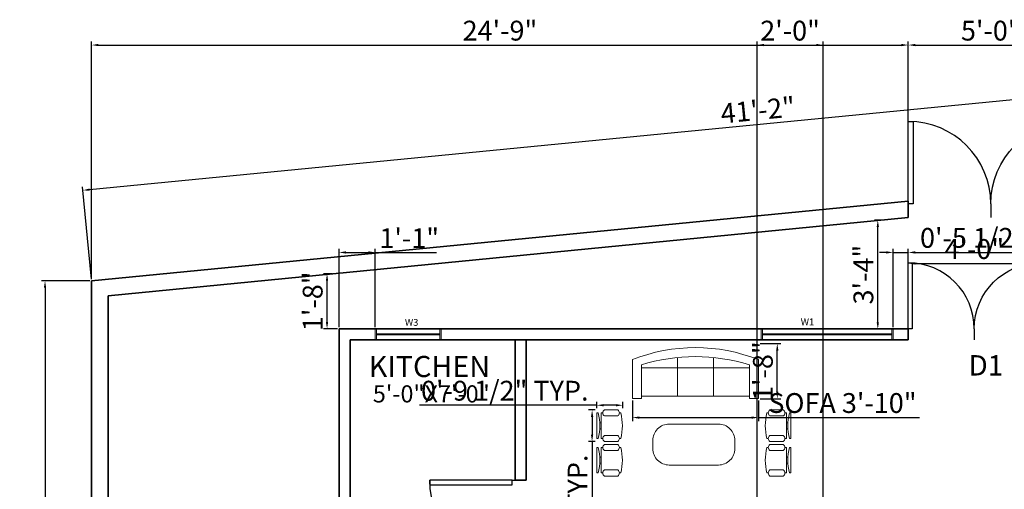
# Model space of a CAD drawing. Units: inches. Extents: x 2165 to 6441, y 2023 to 4425.
# Tile 2 of 4: x 2176 to 2534, y 2281 to 2452. Entities that reach past the tile are written whole.
import ezdxf

# ---------------------------------------------------------------- set-up
doc = ezdxf.new("R2010")
doc.units = ezdxf.units.IN
for name, color, linetype, lineweight in [('A-ANNO-DIMS', 7, 'Continuous', 18), ('A-ANNO-TEXT', 1, 'Continuous', 18), ('A-AREA-IDEN', 1, 'Continuous', 25), ('C-PROP', 7, 'Continuous', 35), ('doors', 5, 'Continuous', 25), ('furniture', 9, 'Continuous', 18), ('walls', 7, 'Continuous', 35), ('windows', 72, 'Continuous', 18)]:
    doc.layers.add(name, color=color, linetype=linetype, lineweight=lineweight)
doc.styles.get("Standard").update_dxf_attribs({"font": 'arial.ttf'})
doc.dimstyles.new('ISO-25', dxfattribs={"dimtxt": 7.203125, "dimasz": 2.5, "dimexe": 1.25, "dimexo": 0.625, "dimtad": 1, "dimdec": 0, "dimlunit": 4, "dimtxsty": 'Standard', "dimcen": 2.5, "dimadec": 0, "dimazin": 0, "dimtfac": 1, "dimtdec": 0, "dimtmove": 0, "dimatfit": 3, "dimfxl": 1, "dimarcsym": 0})

# ---------------------------------------------------------------- blocks, each defined once
blk = doc.blocks.new('*U2')
for p, q in [((0, 0), (0, -5)), ((30, 0), (30, -5))]:
    blk.add_line(p, q)
blk.add_lwpolyline([(0, 0), (0, 30), (1.75, 30), (1.75, 0)], close=True)
blk.add_arc((0, 0), 30, 0, 90)
blk = doc.blocks.new('Sofa - Roundback 7 ft.')
for p, q in [((-36.000027, -34), (-36.000027, -11.4696)), ((-12.00002, -32.4421), (-12.00003, -6.5971)), ((11.99997, -32.4421), (11.99998, -6.5971)), ((35.99998, -34), (35.99998, -11.4696)), ((-35.999844, -13.3819), (35.9998, -13.3819)), ((-36.000027, -32.4421), (35.99998, -32.4421))]:
    blk.add_line(p, q)
for points in [[(-36.000027, -34), (-42.000027, -34), (-42.000027, -8)], [(41.99998, -8), (41.99998, -34), (35.99998, -34)]]:
    blk.add_lwpolyline(points)
for centre, radius, start, end in [((0, -114.25), 114.25, 68.43141, 111.5686), ((-0.00001, -127.1968), 121.1968, 72.72033, 107.2797)]:
    blk.add_arc(centre, radius, start, end)
blk = doc.blocks.new('Chair - Desk')
for p, q in [((-8.5, 0), (-8.5, -1)), ((-8.5, 0), (8.5, 0)), ((8.5, 0), (8.5, -1)), ((-10.5, -5), (-10.5, -14)), ((-8.5, -3), (-8.5, -4)), ((-8.5, -3), (8.5, -3)), ((-6.5, -14), (-6.5, -5)), ((-2, -3), (-2, -1.9355)), ((2, -1.9576), (2, -3)), ((6.5, -5), (6.5, -14)), ((8.5, -3), (8.5, -4)), ((10.5, -14), (10.5, -5)), ((-8.5, -15), (-8.5, -16)), ((8.5, -15), (8.5, -16))]:
    blk.add_line(p, q)
for centre, radius, start, end in [((-8.5, -6.5), 2.5, 36.8699, 143.1301), ((0, 34.625), 36.625, 256.5803, 283.4197), ((8.5, -6.5), 2.5, 36.8699, 143.1301), ((-8.5, -12.5), 2.5, 216.8699, 323.1301), ((0, 19.625), 36.625, 256.5803, 283.4197), ((8.5, -12.5), 2.5, 216.8699, 323.1301)]:
    blk.add_arc(centre, radius, start, end)
blk = doc.blocks.new('*D8')
at = {"layer": 'A-ANNO-DIMS', "color": 0, "lineweight": -2, "transparency": 16777216}
for p, q in [((2693.62, 2405.41), (2690.35, 2438.92)), ((2200.96, 2389.92), (2687.99, 2437.43)), ((2201.62, 2357.41), (2198.35, 2390.92))]:
    blk.add_line(p, q, dxfattribs=at)
at = {"layer": 'A-ANNO-DIMS', "color": 0, "transparency": 16777216}
for points in [[(2687.95, 2437.85), (2688.03, 2437.02), (2690.48, 2437.67)], [(2200.92, 2390.33), (2201, 2389.5), (2198.48, 2389.67)]]:
    blk.add_solid(points, dxfattribs=at)
at = {"layer": 'Defpoints', "color": 0, "transparency": 16777216}
for p in [(2690.48, 2437.67), (2693.68, 2404.78), (2201.68, 2356.78)]:
    blk.add_point(p, dxfattribs=at)
at = {"layer": 'A-ANNO-DIMS', "color": 0, "transparency": 16777216, "insert": (2444.06, 2417.9), "char_height": 7.203, "attachment_point": 5, "rotation": 5.5722}
blk.add_mtext('41\'-2"', dxfattribs=at)
blk = doc.blocks.new('*D10')
at = {"layer": 'A-ANNO-DIMS', "color": 0, "lineweight": -2, "transparency": 16777216}
for p, q in [((2201.06, 2356.78), (2183.49, 2356.78)), ((2184.74, 2354.28), (2184.74, 2059.28)), ((2201.06, 2056.78), (2183.49, 2056.78))]:
    blk.add_line(p, q, dxfattribs=at)
at = {"layer": 'A-ANNO-DIMS', "color": 0, "transparency": 16777216}
for points in [[(2184.32, 2354.28), (2185.15, 2354.28), (2184.74, 2356.78)], [(2184.32, 2059.28), (2185.15, 2059.28), (2184.74, 2056.78)]]:
    blk.add_solid(points, dxfattribs=at)
at = {"layer": 'Defpoints', "color": 0, "transparency": 16777216}
for p in [(2201.68, 2356.78), (2184.74, 2056.78), (2201.68, 2056.78)]:
    blk.add_point(p, dxfattribs=at)
at = {"layer": 'A-ANNO-DIMS', "color": 0, "transparency": 16777216, "insert": (2180.43, 2206.78), "char_height": 7.203, "attachment_point": 5, "rotation": 90}
blk.add_mtext("25'", dxfattribs=at)
blk = doc.blocks.new('*D15')
at = {"layer": 'A-ANNO-DIMS', "color": 0, "lineweight": -2, "transparency": 16777216}
for p, q in [((2289.11, 2359.35), (2286.05, 2359.35)), ((2287.3, 2341.84), (2287.3, 2356.85)), ((2291.06, 2339.34), (2286.05, 2339.34))]:
    blk.add_line(p, q, dxfattribs=at)
at = {"layer": 'A-ANNO-DIMS', "color": 0, "transparency": 16777216}
for points in [[(2286.88, 2356.85), (2287.71, 2356.85), (2287.3, 2359.35)], [(2286.88, 2341.84), (2287.71, 2341.84), (2287.3, 2339.34)]]:
    blk.add_solid(points, dxfattribs=at)
at = {"layer": 'Defpoints', "color": 0, "transparency": 16777216}
for p in [(2287.3, 2359.35), (2289.73, 2359.35), (2291.68, 2339.34)]:
    blk.add_point(p, dxfattribs=at)
at = {"layer": 'A-ANNO-DIMS', "color": 0, "transparency": 16777216, "insert": (2283, 2349.34), "char_height": 7.203, "attachment_point": 5, "rotation": 90}
blk.add_mtext('1\'-8"', dxfattribs=at)
blk = doc.blocks.new('*D16')
at = {"layer": 'A-ANNO-DIMS', "color": 0, "lineweight": -2, "transparency": 16777216}
for p, q in [((2488.7, 2378.82), (2486.34, 2378.82)), ((2487.59, 2341.71), (2487.59, 2376.32)), ((2492.57, 2339.21), (2486.34, 2339.21))]:
    blk.add_line(p, q, dxfattribs=at)
at = {"layer": 'A-ANNO-DIMS', "color": 0, "transparency": 16777216}
for points in [[(2487.17, 2376.32), (2488, 2376.32), (2487.59, 2378.82)], [(2487.17, 2341.71), (2488, 2341.71), (2487.59, 2339.21)]]:
    blk.add_solid(points, dxfattribs=at)
at = {"layer": 'Defpoints', "color": 0, "transparency": 16777216}
for p in [(2487.59, 2378.82), (2489.33, 2378.82), (2493.19, 2339.21)]:
    blk.add_point(p, dxfattribs=at)
at = {"layer": 'A-ANNO-DIMS', "color": 0, "transparency": 16777216, "insert": (2483.28, 2359.02), "char_height": 7.203, "attachment_point": 5, "rotation": 90}
blk.add_mtext('3\'-4"', dxfattribs=at)
blk = doc.blocks.new('WIN-W1-48IN')
for p, q in [((0, 4), (48, 4)), ((0, 0), (0, 4)), ((0.5, 0), (0.5, 4)), ((47.5, 4), (47.5, 0)), ((48, 4), (48, 0)), ((48, 0), (0, 0)), ((0.5, 2.2), (47.5, 2.2)), ((0.5, 1.8), (47.5, 1.8))]:
    blk.add_line(p, q)
blk = doc.blocks.new('WIN-W3-24IN')
for p, q in [((0, 4), (24, 4)), ((0, 0), (0, 4)), ((0.5, 0), (0.5, 4)), ((23.5, 0), (23.5, 4)), ((24, 0), (24, 4)), ((24, 0), (0, 0)), ((23.5, 2.2), (0.5, 2.2)), ((23.5, 1.8), (0.5, 1.8))]:
    blk.add_line(p, q)
blk = doc.blocks.new('*D34')
at = {"layer": 'A-ANNO-DIMS', "color": 0, "lineweight": -2, "transparency": 16777216}
for p, q in [((2384.79, 2309.82), (2382.44, 2309.82)), ((2383.69, 2307.32), (2383.69, 2300.85)), ((2384.79, 2298.35), (2382.44, 2298.35)), ((2383.69, 2298.35), (2383.69, 2194.29))]:
    blk.add_line(p, q, dxfattribs=at)
at = {"layer": 'A-ANNO-DIMS', "color": 0, "transparency": 16777216}
for points in [[(2383.27, 2307.32), (2384.11, 2307.32), (2383.69, 2309.82)], [(2383.27, 2300.85), (2384.11, 2300.85), (2383.69, 2298.35)]]:
    blk.add_solid(points, dxfattribs=at)
at = {"layer": 'Defpoints', "color": 0, "transparency": 16777216}
for p in [(2385.41, 2309.82), (2383.69, 2298.35), (2385.41, 2298.35)]:
    blk.add_point(p, dxfattribs=at)
at = {"layer": 'A-ANNO-DIMS', "color": 0, "transparency": 16777216, "insert": (2379.34, 2245.07), "char_height": 7.2031, "attachment_point": 5, "rotation": 90}
blk.add_mtext('CHAIR 0\'-11 1/2" TYP.', dxfattribs=at)
blk = doc.blocks.new('*D35')
at = {"layer": 'A-ANNO-DIMS', "color": 0, "lineweight": -2, "transparency": 16777216}
for p, q in [((2385.41, 2311.54), (2320.97, 2311.54)), ((2385.41, 2310.44), (2385.41, 2312.79)), ((2392.38, 2311.54), (2387.91, 2311.54)), ((2394.88, 2310.44), (2394.88, 2312.79))]:
    blk.add_line(p, q, dxfattribs=at)
at = {"layer": 'A-ANNO-DIMS', "color": 0, "transparency": 16777216}
for points in [[(2387.91, 2311.95), (2387.91, 2311.12), (2385.41, 2311.54)], [(2392.38, 2311.95), (2392.38, 2311.12), (2394.88, 2311.54)]]:
    blk.add_solid(points, dxfattribs=at)
at = {"layer": 'Defpoints', "color": 0, "transparency": 16777216}
for p in [(2385.41, 2311.54), (2385.41, 2309.82), (2394.88, 2309.82)]:
    blk.add_point(p, dxfattribs=at)
at = {"layer": 'A-ANNO-DIMS', "color": 0, "transparency": 16777216, "insert": (2351.94, 2315.89), "char_height": 7.2031, "attachment_point": 5}
blk.add_mtext('0\'-9 1/2" TYP.', dxfattribs=at)
blk = doc.blocks.new('*D40')
at = {"layer": 'A-ANNO-DIMS', "color": 0, "lineweight": -2, "transparency": 16777216}
for p, q in [((2398.33, 2313.3), (2398.33, 2305.8)), ((2444.16, 2313.3), (2444.16, 2305.8)), ((2400.83, 2307.05), (2441.66, 2307.05)), ((2444.16, 2307.05), (2502.81, 2307.05))]:
    blk.add_line(p, q, dxfattribs=at)
at = {"layer": 'A-ANNO-DIMS', "color": 0, "transparency": 16777216}
for points in [[(2400.83, 2307.47), (2400.83, 2306.64), (2398.33, 2307.05)], [(2441.66, 2307.47), (2441.66, 2306.64), (2444.16, 2307.05)]]:
    blk.add_solid(points, dxfattribs=at)
at = {"layer": 'Defpoints', "color": 0, "transparency": 16777216}
for p in [(2398.33, 2313.93), (2444.16, 2313.93), (2444.16, 2307.05)]:
    blk.add_point(p, dxfattribs=at)
at = {"layer": 'A-ANNO-DIMS', "color": 0, "transparency": 16777216, "insert": (2474.73, 2311.41), "char_height": 7.2031, "attachment_point": 5}
blk.add_mtext('SOFA 3\'-10"', dxfattribs=at)
blk = doc.blocks.new('*D41')
at = {"layer": 'A-ANNO-DIMS', "color": 0, "lineweight": -2, "transparency": 16777216}
for p, q in [((2444.78, 2333.93), (2452.28, 2333.93)), ((2451.03, 2316.43), (2451.03, 2331.43)), ((2444.78, 2313.93), (2452.28, 2313.93))]:
    blk.add_line(p, q, dxfattribs=at)
at = {"layer": 'A-ANNO-DIMS', "color": 0, "transparency": 16777216}
for points in [[(2450.62, 2331.43), (2451.45, 2331.43), (2451.03, 2333.93)], [(2450.62, 2316.43), (2451.45, 2316.43), (2451.03, 2313.93)]]:
    blk.add_solid(points, dxfattribs=at)
at = {"layer": 'Defpoints', "color": 0, "transparency": 16777216}
for p in [(2444.16, 2333.93), (2451.03, 2333.93), (2444.16, 2313.93)]:
    blk.add_point(p, dxfattribs=at)
at = {"layer": 'A-ANNO-DIMS', "color": 0, "transparency": 16777216, "insert": (2446.73, 2323.93), "char_height": 7.203, "attachment_point": 5, "rotation": 90}
blk.add_mtext('1\'-8"', dxfattribs=at)
blk = doc.blocks.new('*D44')
at = {"layer": 'A-ANNO-DIMS', "color": 0, "lineweight": -2, "transparency": 16777216}
for p, q in [((2201.68, 2357.41), (2201.68, 2443.73)), ((2204.18, 2442.48), (2496.18, 2442.48)), ((2498.68, 2386.38), (2498.68, 2443.73))]:
    blk.add_line(p, q, dxfattribs=at)
at = {"layer": 'A-ANNO-DIMS', "color": 0, "transparency": 16777216}
for points in [[(2204.18, 2442.9), (2204.18, 2442.06), (2201.68, 2442.48)], [(2496.18, 2442.9), (2496.18, 2442.06), (2498.68, 2442.48)]]:
    blk.add_solid(points, dxfattribs=at)
at = {"layer": 'Defpoints', "color": 0, "transparency": 16777216}
for p in [(2498.68, 2442.48), (2498.68, 2385.76), (2201.68, 2356.78)]:
    blk.add_point(p, dxfattribs=at)
at = {"layer": 'A-ANNO-DIMS', "color": 0, "transparency": 16777216, "insert": (2350.18, 2446.78), "char_height": 7.203, "attachment_point": 5}
blk.add_mtext('24\'-9"', dxfattribs=at)
blk = doc.blocks.new('*D45')
at = {"layer": 'A-ANNO-DIMS', "color": 0, "lineweight": -2, "transparency": 16777216}
for p, q in [((2498.68, 2415.36), (2498.68, 2443.73)), ((2501.18, 2442.48), (2556.18, 2442.48)), ((2558.68, 2415.36), (2558.68, 2443.73))]:
    blk.add_line(p, q, dxfattribs=at)
at = {"layer": 'A-ANNO-DIMS', "color": 0, "transparency": 16777216}
for points in [[(2501.18, 2442.9), (2501.18, 2442.06), (2498.68, 2442.48)], [(2556.18, 2442.9), (2556.18, 2442.06), (2558.68, 2442.48)]]:
    blk.add_solid(points, dxfattribs=at)
at = {"layer": 'Defpoints', "color": 0, "transparency": 16777216}
for p in [(2558.68, 2442.48), (2498.68, 2414.73), (2558.68, 2414.73)]:
    blk.add_point(p, dxfattribs=at)
at = {"layer": 'A-ANNO-DIMS', "color": 0, "transparency": 16777216, "insert": (2528.68, 2446.78), "char_height": 7.203, "attachment_point": 5}
blk.add_mtext('5\'-0"', dxfattribs=at)
blk = doc.blocks.new('*D46')
at = {"layer": 'A-ANNO-DIMS', "color": 0, "lineweight": -2, "transparency": 16777216}
for p, q in [((2498.68, 2335.97), (2498.68, 2364.34)), ((2546.68, 2335.97), (2546.68, 2364.34)), ((2501.18, 2363.09), (2544.18, 2363.09))]:
    blk.add_line(p, q, dxfattribs=at)
at = {"layer": 'A-ANNO-DIMS', "color": 0, "transparency": 16777216}
for points in [[(2501.18, 2363.51), (2501.18, 2362.67), (2498.68, 2363.09)], [(2544.18, 2363.51), (2544.18, 2362.67), (2546.68, 2363.09)]]:
    blk.add_solid(points, dxfattribs=at)
at = {"layer": 'Defpoints', "color": 0, "transparency": 16777216}
for p in [(2546.68, 2363.09), (2498.68, 2335.34), (2546.68, 2335.34)]:
    blk.add_point(p, dxfattribs=at)
at = {"layer": 'A-ANNO-DIMS', "color": 0, "transparency": 16777216, "insert": (2522.68, 2367.39), "char_height": 7.203, "attachment_point": 5}
blk.add_mtext('4\'-0"', dxfattribs=at)
blk = doc.blocks.new('*D54')
at = {"layer": 'A-ANNO-DIMS', "color": 0, "lineweight": -2, "transparency": 16777216}
for p, q in [((2443.68, 2153.41), (2443.68, 2443.73)), ((2446.18, 2442.48), (2465.18, 2442.48)), ((2467.68, 2173.28), (2467.68, 2443.73))]:
    blk.add_line(p, q, dxfattribs=at)
at = {"layer": 'A-ANNO-DIMS', "color": 0, "transparency": 16777216}
for points in [[(2446.18, 2442.9), (2446.18, 2442.06), (2443.68, 2442.48)], [(2465.18, 2442.9), (2465.18, 2442.06), (2467.68, 2442.48)]]:
    blk.add_solid(points, dxfattribs=at)
at = {"layer": 'Defpoints', "color": 0, "transparency": 16777216}
for p in [(2467.68, 2442.48), (2467.68, 2172.66), (2443.68, 2152.78)]:
    blk.add_point(p, dxfattribs=at)
at = {"layer": 'A-ANNO-DIMS', "color": 0, "transparency": 16777216, "insert": (2455.68, 2446.78), "char_height": 7.203, "attachment_point": 5}
blk.add_mtext('2\'-0"', dxfattribs=at)
blk = doc.blocks.new('*D56')
at = {"layer": 'A-ANNO-DIMS', "color": 0, "lineweight": -2, "transparency": 16777216}
for p, q in [((2291.68, 2339.97), (2291.68, 2368.34)), ((2294.18, 2367.09), (2302.33, 2367.09)), ((2304.83, 2339.97), (2304.83, 2368.34)), ((2304.83, 2367.09), (2327.05, 2367.09))]:
    blk.add_line(p, q, dxfattribs=at)
at = {"layer": 'A-ANNO-DIMS', "color": 0, "transparency": 16777216}
for points in [[(2294.18, 2367.51), (2294.18, 2366.67), (2291.68, 2367.09)], [(2302.33, 2367.51), (2302.33, 2366.67), (2304.83, 2367.09)]]:
    blk.add_solid(points, dxfattribs=at)
at = {"layer": 'Defpoints', "color": 0, "transparency": 16777216}
for p in [(2304.83, 2367.09), (2291.68, 2339.34), (2304.83, 2339.34)]:
    blk.add_point(p, dxfattribs=at)
at = {"layer": 'A-ANNO-DIMS', "color": 0, "transparency": 16777216, "insert": (2317.19, 2371.33), "char_height": 7.203, "attachment_point": 5}
blk.add_mtext('1\'-1"', dxfattribs=at)
blk = doc.blocks.new('*D57')
at = {"layer": 'A-ANNO-DIMS', "color": 0, "lineweight": -2, "transparency": 16777216}
for p, q in [((2490.69, 2367.09), (2488.19, 2367.09)), ((2493.19, 2339.97), (2493.19, 2368.34)), ((2493.19, 2367.09), (2498.68, 2367.09)), ((2498.68, 2339.97), (2498.68, 2368.34)), ((2501.18, 2367.09), (2540.87, 2367.09))]:
    blk.add_line(p, q, dxfattribs=at)
at = {"layer": 'A-ANNO-DIMS', "color": 0, "transparency": 16777216}
for points in [[(2490.69, 2367.51), (2490.69, 2366.67), (2493.19, 2367.09)], [(2501.18, 2367.51), (2501.18, 2366.67), (2498.68, 2367.09)]]:
    blk.add_solid(points, dxfattribs=at)
at = {"layer": 'Defpoints', "color": 0, "transparency": 16777216}
for p in [(2498.68, 2367.09), (2493.19, 2339.34), (2498.68, 2339.34)]:
    blk.add_point(p, dxfattribs=at)
at = {"layer": 'A-ANNO-DIMS', "color": 0, "transparency": 16777216, "insert": (2522.28, 2371.44), "char_height": 7.203, "attachment_point": 5}
blk.add_mtext('0\'-5 1/2"', dxfattribs=at)

msp = doc.modelspace()

# ---------------------------------------------------------------- linework, layer by layer
at = {"layer": 'C-PROP'}
for p, q in [((2201.68, 2356.78), (2498.68, 2385.76)), ((2498.68, 2379.73), (2498.68, 2385.76)), ((2498.68, 2379.73), (2498.68, 2384.73)), ((2207.68, 2351.34), (2498.68, 2379.73)), ((2201.68, 2056.78), (2201.68, 2356.78)), ((2207.68, 2062.78), (2207.68, 2351.34))]:
    msp.add_line(p, q, dxfattribs=at)
at = {"layer": 'furniture'}
msp.add_lwpolyline([(2429.62, 2304.7, -0.414214), (2435.58, 2298.74), (2435.58, 2295.76, -0.414214), (2429.62, 2289.81), (2411.74, 2289.81, -0.414214), (2405.79, 2295.76), (2405.79, 2298.74, -0.414214), (2411.74, 2304.7)], format="xyb", close=True, dxfattribs=at)
at = {"layer": 'walls'}
for p, q in [((2291.68, 2074.78), (2291.68, 2339.34)), ((2498.68, 2339.34), (2291.68, 2339.34)), ((2498.68, 2335.34), (2498.68, 2339.34)), ((2295.68, 2078.78), (2295.68, 2335.34)), ((2498.68, 2335.34), (2295.68, 2335.34)), ((2355.68, 2284.34), (2355.68, 2335.34)), ((2359.68, 2284.34), (2359.68, 2335.34)), ((2359.68, 2284.34), (2355.68, 2284.34))]:
    msp.add_line(p, q, dxfattribs=at)

# ---------------------------------------------------------------- block references
at = {"layer": 'doors'}
msp.add_blockref('*U2', (2498.68, 2384.73), dxfattribs=at)
at = {"layer": 'doors', "xscale": -1}
msp.add_blockref('*U2', (2558.68, 2384.73), dxfattribs=at)
at = {"layer": 'doors', "yscale": 0.8, "zscale": 0.8}
for p, xscale in [((2498.68, 2339.34), 0.8), ((2546.68, 2339.34), -0.8)]:
    msp.add_blockref('*U2', p, dxfattribs=dict(at, xscale=xscale))
at = {"layer": 'doors', "xscale": -1, "rotation": 90}
msp.add_blockref('*U2', (2354.68, 2284.34), dxfattribs=at)
at = {"layer": 'furniture', "xscale": 0.5455519184629141, "yscale": 0.5455519184629141, "zscale": 0.5455519184629141}
msp.add_blockref('Sofa - Roundback 7 ft.', (2421.24, 2332.48), dxfattribs=at)
at = {"layer": 'furniture', "yscale": 0.5460527943098772, "zscale": 0.5460527943098772}
for p, xscale, rotation in [((2385.41, 2304.08), -0.5460527943098772, 90), ((2455.97, 2304.08), 0.5460527943098772, 270), ((2385.41, 2291.55), -0.5460527943098772, 90), ((2455.97, 2291.55), 0.5460527943098772, 270)]:
    msp.add_blockref('Chair - Desk', p, dxfattribs=dict(at, xscale=xscale, rotation=rotation))
at = {"layer": 'windows'}
for name, p in [('WIN-W3-24IN', (2304.83, 2335.34)), ('WIN-W1-48IN', (2445.19, 2335.34))]:
    msp.add_blockref(name, p, dxfattribs=at)

# ---------------------------------------------------------------- texts
at = {"layer": 'A-ANNO-TEXT', "attachment_point": 1}
for s, width, gutter_width, insert, char_height in [('W3', 0.1172, 12.5, (2315.62, 2342.91), 2.5), ('W1', 0.1172, 12.5, (2459.57, 2343.08), 2.5), ('D1', 3.6504, 37, (2520.62, 2329.75), 7.4)]:
    msp.add_mtext_dynamic_manual_height_columns(s, width=width, gutter_width=gutter_width, heights=[0], dxfattribs=dict(at, insert=insert, char_height=char_height))
at = {"layer": 'A-AREA-IDEN', "attachment_point": 1}
for s, width, gutter_width, insert, char_height in [('KITCHEN', 2.1423, 38.36, (2302.47, 2329.46), 7.672), ('5\'-0"X7\'-0"', 0.6986, 31.22, (2303.95, 2318.79), 6.2446)]:
    msp.add_mtext_dynamic_manual_height_columns(s, width=width, gutter_width=gutter_width, heights=[0], dxfattribs=dict(at, insert=insert, char_height=char_height))

# ---------------------------------------------------------------- dimensions: what is measured, and where the dimension line sits
at = {"layer": 'A-ANNO-DIMS'}
for base, p1, p2, picture, middle in [((2498.68, 2442.48), (2201.68, 2356.78), (2498.68, 2385.76), '*D44', (2350.18, 2446.78)), ((2467.68, 2442.48), (2443.68, 2152.78), (2467.68, 2172.66), '*D54', (2455.68, 2446.78)), ((2558.68, 2442.48), (2498.68, 2414.73), (2558.68, 2414.73), '*D45', (2528.68, 2446.78)), ((2498.68, 2367.09), (2493.19, 2339.34), (2498.68, 2339.34), '*D57', (2522.28, 2371.44)), ((2304.8275, 2367.091), (2291.684, 2339.341), (2304.8275, 2339.341), '*D56', (2317.1874, 2371.3323)), ((2546.68, 2363.09), (2498.68, 2335.34), (2546.68, 2335.34), '*D46', (2522.68, 2367.39))]:
    dim = msp.add_linear_dim(base=base, p1=p1, p2=p2, dimstyle='ISO-25', override={"dimdec": 1, "dimlfac": 1, "dimrnd": 0, "dimzin": 1, "dimdsep": 46, "dimlunit": 4, "dimfrac": 2}, dxfattribs=at)
    dim.commit()
    dim.dimension.update_dxf_attribs({"geometry": picture, "text_midpoint": middle})
dim = msp.add_aligned_dim(p1=(2201.68, 2356.78), p2=(2693.68, 2404.78), distance=33.05, dimstyle='ISO-25', override={"dimclrd": 0, "dimclre": 0, "dimclrt": 0}, dxfattribs=at)
dim.commit()
dim.dimension.update_dxf_attribs({"geometry": '*D8', "text_midpoint": (2444.06, 2417.9)})
for base, p1, p2, override, picture, middle in [((2487.59, 2378.82), (2493.19, 2339.21), (2489.33, 2378.82), {"dimclrd": 0, "dimclre": 0, "dimclrt": 0}, '*D16', (2483.28, 2359.02)), ((2287.3, 2359.35), (2291.68, 2339.34), (2289.73, 2359.35), {"dimclrd": 0, "dimclre": 0, "dimclrt": 0}, '*D15', (2283, 2349.34)), ((2451.03, 2333.93), (2444.16, 2313.93), (2444.16, 2333.93), {"dimdec": 1, "dimlfac": 1, "dimrnd": 0, "dimzin": 1, "dimdsep": 46, "dimlunit": 4, "dimfrac": 2}, '*D41', (2446.73, 2323.93))]:
    dim = msp.add_linear_dim(base=base, p1=p1, p2=p2, angle=90, dimstyle='ISO-25', override=override, dxfattribs=at)
    dim.commit()
    dim.dimension.update_dxf_attribs({"geometry": picture, "text_midpoint": middle})
dim = msp.add_linear_dim(base=(2184.74, 2056.78), p1=(2201.68, 2356.78), p2=(2201.68, 2056.78), angle=90, dimstyle='ISO-25', override={"dimclrd": 0, "dimclre": 0, "dimclrt": 0}, dxfattribs=at)
dim.commit()
dim.dimension.update_dxf_attribs({"geometry": '*D10', "text_midpoint": (2184.74, 2206.78), "dimtype": 160})
for base, p1, p2, angle, text, picture, middle in [((2385.41, 2311.54), (2394.88, 2309.82), (2385.41, 2309.82), 180, '<> TYP.', '*D35', (2351.94, 2315.89)), ((2383.69, 2298.35), (2385.41, 2309.82), (2385.41, 2298.35), 270, 'CHAIR <> TYP.', '*D34', (2379.34, 2245.07))]:
    dim = msp.add_linear_dim(base=base, p1=p1, p2=p2, angle=angle, text=text, dimstyle='ISO-25', override={"dimdec": 1, "dimlfac": 1, "dimrnd": 0, "dimzin": 1, "dimdsep": 46, "dimlunit": 4, "dimfrac": 2}, dxfattribs=at)
    dim.commit()
    dim.dimension.update_dxf_attribs({"geometry": picture, "text_midpoint": middle})
dim = msp.add_linear_dim(base=(2444.16, 2307.05), p1=(2398.33, 2313.93), p2=(2444.16, 2313.93), text='SOFA <>', dimstyle='ISO-25', override={"dimdec": 1, "dimlfac": 1, "dimrnd": 0, "dimzin": 1, "dimdsep": 46, "dimlunit": 4, "dimfrac": 2}, dxfattribs=at)
dim.commit()
dim.dimension.update_dxf_attribs({"geometry": '*D40', "text_midpoint": (2474.73, 2311.41)})

doc.saveas('drawing.dxf')
